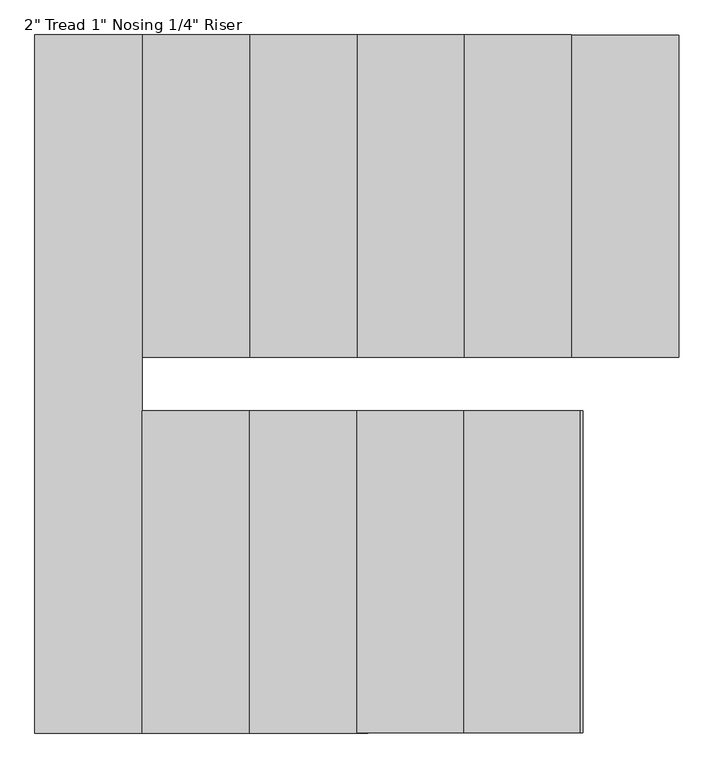
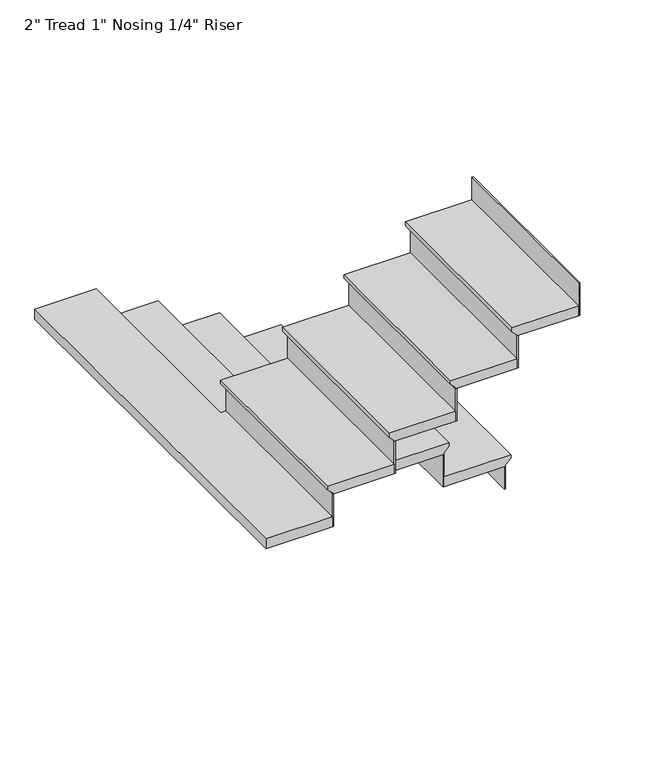
"""IFC4 building model written with IfcOpenShell, lengths in millimetres: stair flight geometry."""

from ifc_helpers import new_model, si_unit, origin, place, context, project, spatial, faceted_brep, source, transform, mapped, element, save


def stair_flight_f33635a8(model_context):
    return source(origin(), model_context, "Body", "Brep", [
        faceted_brep([(3327.4, 3340.1, 9294.2833333), (3327.4, 3340.1, 9313.3333333), (3327.4, 2425.7, 9313.3333333), (3327.4, 2425.7, 9294.2833333), (3302.0, 3340.1, 9268.8833333), (3302.0, 2425.7, 9268.8833333), (2997.2, 3340.1, 9313.3333333), (2997.2, 2425.7, 9313.3333333), (3302.0, 2425.7, 9262.5333333), (2997.2, 2425.7, 9262.5333333), (2997.2, 3340.1, 9262.5333333), (3302.0, 3340.1, 9262.5333333)], [[[0, 1, 2, 3]], [[4, 0, 3, 5]], [[2, 1, 6, 7]], [[8, 9, 10, 11]], [[2, 7, 9, 8, 5, 3]], [[8, 11, 4, 5]], [[6, 1, 0, 4, 11, 10]], [[7, 6, 10, 9]]]),
        faceted_brep([(3302.0, 3340.1, 9262.5333333), (3302.0, 3340.1, 9144.0), (3295.65, 3340.1, 9144.0), (3295.65, 3340.1, 9262.5333333), (3302.0, 2425.7, 9262.5333333), (3295.65, 2425.7, 9262.5333333), (3295.65, 2425.7, 9144.0), (3302.0, 2425.7, 9144.0)], [[[0, 1, 2, 3]], [[4, 5, 6, 7]], [[1, 0, 4, 7]], [[2, 1, 7, 6]], [[3, 2, 6, 5]], [[0, 3, 5, 4]]]),
        faceted_brep([(2997.2, 3340.1, 9431.8666667), (2997.2, 3340.1, 9262.5333333), (2990.85, 3340.1, 9262.5333333), (2990.85, 3340.1, 9431.8666667), (2997.2, 2425.7, 9431.8666667), (2990.85, 2425.7, 9431.8666667), (2990.85, 2425.7, 9262.5333333), (2997.2, 2425.7, 9262.5333333)], [[[0, 1, 2, 3]], [[4, 5, 6, 7]], [[1, 0, 4, 7]], [[2, 1, 7, 6]], [[3, 2, 6, 5]], [[0, 3, 5, 4]]]),
        faceted_brep([(3022.6, 2425.7, 9482.6666667), (3022.6, 3340.1, 9482.6666667), (2692.4, 3340.1, 9482.6666667), (2692.4, 2425.7, 9482.6666667), (2997.2, 2425.7, 9431.8666667), (2692.4, 2425.7, 9431.8666667), (2692.4, 3340.1, 9431.8666667), (2997.2, 3340.1, 9431.8666667), (2997.2, 2425.7, 9438.2166667), (3022.6, 2425.7, 9463.6166667), (2997.2, 3340.1, 9438.2166667), (3022.6, 3340.1, 9463.6166667)], [[[0, 1, 2, 3]], [[4, 5, 6, 7]], [[0, 3, 5, 4, 8, 9]], [[4, 7, 10, 8]], [[2, 1, 11, 10, 7, 6]], [[3, 2, 6, 5]], [[11, 1, 0, 9]], [[10, 11, 9, 8]]]),
        faceted_brep([(2692.4, 3340.1, 9601.2), (2692.4, 3340.1, 9431.8666667), (2686.05, 3340.1, 9431.8666667), (2686.05, 3340.1, 9601.2), (2692.4, 2425.7, 9601.2), (2686.05, 2425.7, 9601.2), (2686.05, 2425.7, 9431.8666667), (2692.4, 2425.7, 9431.8666667)], [[[0, 1, 2, 3]], [[4, 5, 6, 7]], [[1, 0, 4, 7]], [[2, 1, 7, 6]], [[3, 2, 6, 5]], [[0, 3, 5, 4]]]),
        faceted_brep([(2717.8, 2425.7, 9652.0), (2717.8, 3340.1, 9652.0), (2387.6, 3340.1, 9652.0), (2387.6, 2425.7, 9652.0), (2692.4, 2425.7, 9601.2), (2387.6, 2425.7, 9601.2), (2387.6, 3340.1, 9601.2), (2692.4, 3340.1, 9601.2), (2692.4, 2425.7, 9607.55), (2717.8, 2425.7, 9632.95), (2692.4, 3340.1, 9607.55), (2717.8, 3340.1, 9632.95)], [[[0, 1, 2, 3]], [[4, 5, 6, 7]], [[0, 3, 5, 4, 8, 9]], [[4, 7, 10, 8]], [[2, 1, 11, 10, 7, 6]], [[3, 2, 6, 5]], [[11, 1, 0, 9]], [[10, 11, 9, 8]]]),
        faceted_brep([(2387.6, 3340.1, 9770.5333333), (2387.6, 3340.1, 9601.2), (2381.25, 3340.1, 9601.2), (2381.25, 3340.1, 9770.5333333), (2387.6, 2425.7, 9770.5333333), (2381.25, 2425.7, 9770.5333333), (2381.25, 2425.7, 9601.2), (2387.6, 2425.7, 9601.2)], [[[0, 1, 2, 3]], [[4, 5, 6, 7]], [[1, 0, 4, 7]], [[2, 1, 7, 6]], [[3, 2, 6, 5]], [[0, 3, 5, 4]]]),
        faceted_brep([(2413.0, 2425.7, 9821.3333333), (2413.0, 3340.1, 9821.3333333), (2082.8, 3340.1, 9821.3333333), (2082.8, 2425.7, 9821.3333333), (2387.6, 2425.7, 9770.5333333), (2082.8, 2425.7, 9770.5333333), (2082.8, 3340.1, 9770.5333333), (2387.6, 3340.1, 9770.5333333), (2387.6, 2425.7, 9776.8833333), (2413.0, 2425.7, 9802.2833333), (2387.6, 3340.1, 9776.8833333), (2413.0, 3340.1, 9802.2833333)], [[[0, 1, 2, 3]], [[4, 5, 6, 7]], [[0, 3, 5, 4, 8, 9]], [[4, 7, 10, 8]], [[2, 1, 11, 10, 7, 6]], [[3, 2, 6, 5]], [[11, 1, 0, 9]], [[10, 11, 9, 8]]]),
        faceted_brep([(2082.8, 3340.1, 9939.8666667), (2082.8, 3340.1, 9770.5333333), (2076.45, 3340.1, 9770.5333333), (2076.45, 3340.1, 9939.8666667), (2082.8, 2425.7, 9939.8666667), (2076.45, 2425.7, 9939.8666667), (2076.45, 2425.7, 9770.5333333), (2082.8, 2425.7, 9770.5333333)], [[[0, 1, 2, 3]], [[4, 5, 6, 7]], [[1, 0, 4, 7]], [[2, 1, 7, 6]], [[3, 2, 6, 5]], [[0, 3, 5, 4]]]),
        faceted_brep([(2108.2, 2425.7, 9990.6666667), (2108.2, 3340.1, 9990.6666667), (1778.0, 3340.1, 9990.6666667), (1778.0, 2425.7, 9990.6666667), (2082.8, 2425.7, 9939.8666667), (1778.0, 2425.7, 9939.8666667), (1778.0, 3340.1, 9939.8666667), (2082.8, 3340.1, 9939.8666667), (2082.8, 2425.7, 9946.2166667), (2108.2, 2425.7, 9971.6166667), (2082.8, 3340.1, 9946.2166667), (2108.2, 3340.1, 9971.6166667)], [[[0, 1, 2, 3]], [[4, 5, 6, 7]], [[0, 3, 5, 4, 8, 9]], [[4, 7, 10, 8]], [[2, 1, 11, 10, 7, 6]], [[3, 2, 6, 5]], [[11, 1, 0, 9]], [[10, 11, 9, 8]]]),
        faceted_brep([(1778.0, 3340.1, 10109.2), (1778.0, 3340.1, 9939.8666667), (1771.65, 3340.1, 9939.8666667), (1771.65, 3340.1, 10109.2), (1778.0, 2425.7, 10109.2), (1771.65, 2425.7, 10109.2), (1771.65, 2425.7, 9939.8666667), (1778.0, 2425.7, 9939.8666667)], [[[0, 1, 2, 3]], [[4, 5, 6, 7]], [[1, 0, 4, 7]], [[2, 1, 7, 6]], [[3, 2, 6, 5]], [[0, 3, 5, 4]]]),
        faceted_brep([(1828.8, 2273.3, 10160.0), (1803.4, 2273.3, 10160.0), (1803.4, 3340.1, 10160.0), (1498.6, 3340.1, 10160.0), (1498.6, 1358.9, 10160.0), (1828.8, 1358.9, 10160.0), (1803.4, 2273.3, 10109.2), (1828.8, 2273.3, 10109.2), (1828.8, 1358.9, 10109.2), (1498.6, 1358.9, 10109.2), (1498.6, 3340.1, 10109.2), (1778.0, 3340.1, 10109.2), (1778.0, 2425.7, 10109.2), (1803.4, 2425.7, 10109.2), (1803.4, 2425.7, 10140.95), (1803.4, 3340.1, 10140.95), (1778.0, 2425.7, 10115.55), (1778.0, 3340.1, 10115.55)], [[[0, 1, 2, 3, 4, 5]], [[6, 7, 8, 9, 10, 11, 12, 13]], [[1, 0, 7, 6]], [[2, 1, 6, 13, 14, 15]], [[13, 12, 16, 14]], [[12, 11, 17, 16]], [[3, 2, 15, 17, 11, 10]], [[4, 3, 10, 9]], [[5, 4, 9, 8]], [[0, 5, 8, 7]], [[17, 15, 14, 16]]]),
        faceted_brep([(1828.8, 1358.9, 10278.5333333), (1828.8, 1358.9, 10109.2), (1835.15, 1358.9, 10109.2), (1835.15, 1358.9, 10278.5333333), (1828.8, 2273.3, 10278.5333333), (1835.15, 2273.3, 10278.5333333), (1835.15, 2273.3, 10109.2), (1828.8, 2273.3, 10109.2)], [[[0, 1, 2, 3]], [[4, 5, 6, 7]], [[1, 0, 4, 7]], [[2, 1, 7, 6]], [[3, 2, 6, 5]], [[0, 3, 5, 4]]]),
        faceted_brep([(1803.4, 2273.3, 10329.3333333), (1803.4, 1358.9, 10329.3333333), (2133.6, 1358.9, 10329.3333333), (2133.6, 2273.3, 10329.3333333), (1828.8, 2273.3, 10278.5333333), (2133.6, 2273.3, 10278.5333333), (2133.6, 1358.9, 10278.5333333), (1828.8, 1358.9, 10278.5333333), (1828.8, 2273.3, 10284.8833333), (1803.4, 2273.3, 10310.2833333), (1828.8, 1358.9, 10284.8833333), (1803.4, 1358.9, 10310.2833333)], [[[0, 1, 2, 3]], [[4, 5, 6, 7]], [[0, 3, 5, 4, 8, 9]], [[4, 7, 10, 8]], [[2, 1, 11, 10, 7, 6]], [[3, 2, 6, 5]], [[11, 1, 0, 9]], [[10, 11, 9, 8]]]),
        faceted_brep([(2133.6, 1358.9, 10447.8666667), (2133.6, 1358.9, 10278.5333333), (2139.95, 1358.9, 10278.5333333), (2139.95, 1358.9, 10447.8666667), (2133.6, 2273.3, 10447.8666667), (2139.95, 2273.3, 10447.8666667), (2139.95, 2273.3, 10278.5333333), (2133.6, 2273.3, 10278.5333333)], [[[0, 1, 2, 3]], [[4, 5, 6, 7]], [[1, 0, 4, 7]], [[2, 1, 7, 6]], [[3, 2, 6, 5]], [[0, 3, 5, 4]]]),
        faceted_brep([(2108.2, 2273.3, 10498.6666667), (2108.2, 1358.9, 10498.6666667), (2438.4, 1358.9, 10498.6666667), (2438.4, 2273.3, 10498.6666667), (2133.6, 2273.3, 10447.8666667), (2438.4, 2273.3, 10447.8666667), (2438.4, 1358.9, 10447.8666667), (2133.6, 1358.9, 10447.8666667), (2133.6, 2273.3, 10454.2166667), (2108.2, 2273.3, 10479.6166667), (2133.6, 1358.9, 10454.2166667), (2108.2, 1358.9, 10479.6166667)], [[[0, 1, 2, 3]], [[4, 5, 6, 7]], [[0, 3, 5, 4, 8, 9]], [[4, 7, 10, 8]], [[2, 1, 11, 10, 7, 6]], [[3, 2, 6, 5]], [[11, 1, 0, 9]], [[10, 11, 9, 8]]]),
        faceted_brep([(2438.4, 1358.9, 10617.2), (2438.4, 1358.9, 10447.8666667), (2444.75, 1358.9, 10447.8666667), (2444.75, 1358.9, 10617.2), (2438.4, 2273.3, 10617.2), (2444.75, 2273.3, 10617.2), (2444.75, 2273.3, 10447.8666667), (2438.4, 2273.3, 10447.8666667)], [[[0, 1, 2, 3]], [[4, 5, 6, 7]], [[1, 0, 4, 7]], [[2, 1, 7, 6]], [[3, 2, 6, 5]], [[0, 3, 5, 4]]]),
        faceted_brep([(2413.0, 2273.3, 10668.0), (2413.0, 1358.9, 10668.0), (2743.2, 1358.9, 10668.0), (2743.2, 2273.3, 10668.0), (2438.4, 2273.3, 10617.2), (2743.2, 2273.3, 10617.2), (2743.2, 1358.9, 10617.2), (2438.4, 1358.9, 10617.2), (2438.4, 2273.3, 10623.55), (2413.0, 2273.3, 10648.95), (2438.4, 1358.9, 10623.55), (2413.0, 1358.9, 10648.95)], [[[0, 1, 2, 3]], [[4, 5, 6, 7]], [[0, 3, 5, 4, 8, 9]], [[4, 7, 10, 8]], [[2, 1, 11, 10, 7, 6]], [[3, 2, 6, 5]], [[11, 1, 0, 9]], [[10, 11, 9, 8]]]),
        faceted_brep([(2743.2, 1358.9, 10786.5333333), (2743.2, 1358.9, 10617.2), (2749.55, 1358.9, 10617.2), (2749.55, 1358.9, 10786.5333333), (2743.2, 2273.3, 10786.5333333), (2749.55, 2273.3, 10786.5333333), (2749.55, 2273.3, 10617.2), (2743.2, 2273.3, 10617.2)], [[[0, 1, 2, 3]], [[4, 5, 6, 7]], [[1, 0, 4, 7]], [[2, 1, 7, 6]], [[3, 2, 6, 5]], [[0, 3, 5, 4]]]),
        faceted_brep([(3048.0, 1358.9, 10955.8666667), (3048.0, 1358.9, 10786.5333333), (3054.35, 1358.9, 10786.5333333), (3054.35, 1358.9, 10955.8666667), (3048.0, 2273.3, 10955.8666667), (3054.35, 2273.3, 10955.8666667), (3054.35, 2273.3, 10786.5333333), (3048.0, 2273.3, 10786.5333333)], [[[0, 1, 2, 3]], [[4, 5, 6, 7]], [[1, 0, 4, 7]], [[2, 1, 7, 6]], [[3, 2, 6, 5]], [[0, 3, 5, 4]]]),
        faceted_brep([(2717.8, 2273.3, 10837.3333333), (2717.8, 1358.9, 10837.3333333), (3048.0, 1358.9, 10837.3333333), (3048.0, 2273.3, 10837.3333333), (2743.2, 2273.3, 10786.5333333), (3048.0, 2273.3, 10786.5333333), (3048.0, 1358.9, 10786.5333333), (2743.2, 1358.9, 10786.5333333), (2743.2, 2273.3, 10792.8833333), (2717.8, 2273.3, 10818.2833333), (2743.2, 1358.9, 10792.8833333), (2717.8, 1358.9, 10818.2833333)], [[[0, 1, 2, 3]], [[4, 5, 6, 7]], [[0, 3, 5, 4, 8, 9]], [[4, 7, 10, 8]], [[2, 1, 11, 10, 7, 6]], [[3, 2, 6, 5]], [[11, 1, 0, 9]], [[10, 11, 9, 8]]]),
    ])


if __name__ == "__main__":
    model = new_model("IFC4")
    model_context = context("Model", 3, world=origin())
    ifc_project = project(units=[si_unit("LENGTHUNIT", "METRE", prefix="MILLI")], contexts=[model_context])
    site = spatial("IfcSite", under=ifc_project)
    building = spatial("IfcBuilding", under=site)
    placement = place(None, origin())
    stair_flight_shape = stair_flight_f33635a8(model_context)
    element("IfcStairFlight", 1, ObjectType="2\" Tread 1\" Nosing 1/4\" Riser", at=placement, inside=building, context=model_context, shape_type="MappedRepresentation", body=[
        mapped(stair_flight_shape, transform((0.0, 0.0, 0.0), x_axis=(1.0, 0.0, 0.0), y_axis=(0.0, 1.0, 0.0), z_axis=(0.0, 0.0, 1.0))),
    ])
    save(model, "model.ifc")
